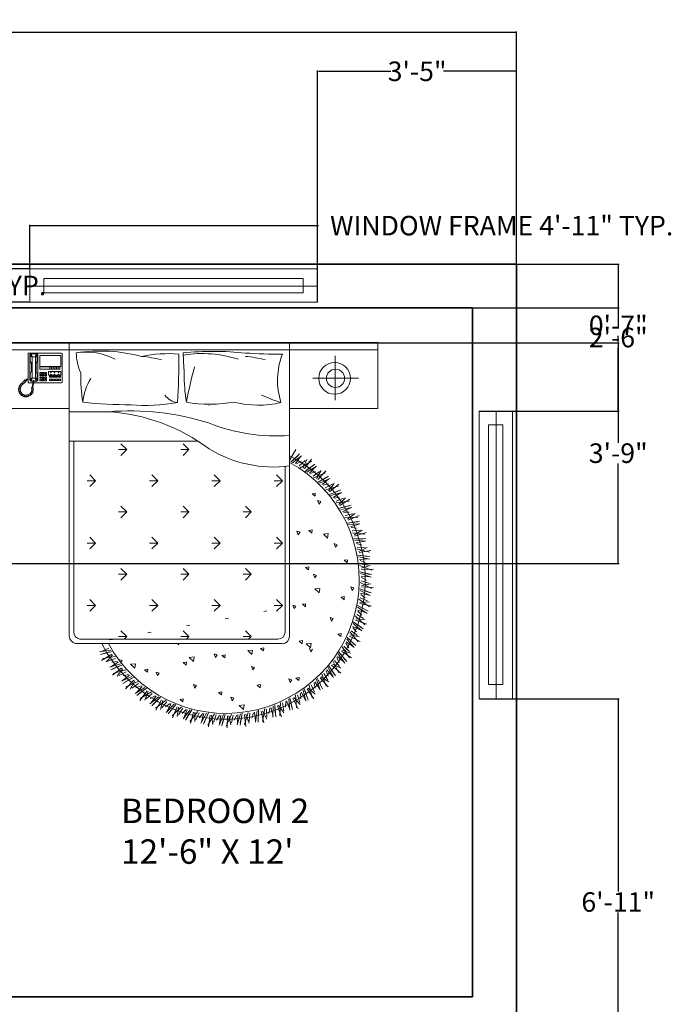
# Model space of a CAD drawing. Units: inches. Extents: x 311 to 754, y 60 to 497.
# Tile 11 of 11: x 621 to 754, y 296 to 497. Entities that reach past the tile are written whole.
import ezdxf

# ---------------------------------------------------------------- set-up
doc = ezdxf.new("R2010")
doc.units = ezdxf.units.IN
doc.header["$MEASUREMENT"] = 0
for name, color, linetype, lineweight in [('A-ANNO-DIMS', 2, 'Continuous', 18), ('A-AREA-IDEN', 1, 'Continuous', 18), ('A-WALL', 7, 'Continuous', 35), ('beds', 70, 'Continuous', 13), ('windows', 120, 'Continuous', 18)]:
    doc.layers.add(name, color=color, linetype=linetype, lineweight=lineweight)
doc.styles.get("Standard").update_dxf_attribs({"font": 'arial.ttf'})
doc.dimstyles.get("Standard").update_dxf_attribs({"dimtxt": 4, "dimasz": 0.18, "dimexe": 0.18, "dimexo": 0.0625, "dimgap": 0.09, "dimtad": 0, "dimtih": 1, "dimtoh": 1, "dimdec": 0, "dimrnd": 6, "dimzin": 0, "dimdsep": 46, "dimlunit": 3, "dimtxsty": 'Standard', "dimcen": 0.09, "dimadec": 0, "dimazin": 0, "dimtfac": 1, "dimtdec": 0, "dimtofl": 0, "dimtmove": 0, "dimatfit": 3, "dimfxl": 1, "dimtolj": 1, "dimtzin": 0, "dimarcsym": 0})

# ---------------------------------------------------------------- blocks, each defined once
blk = doc.blocks.new('A$C57792D97')
for p, q in [((0.6, 2.6235), (0, 2.6235)), ((0, 2.6235), (0, 2.1735)), ((2.1, 2.6235), (0.6, 2.6235)), ((0.6, 2.6235), (0.6, 0.6235)), ((0.6, 0.6235), (0.6, 2.6235)), ((0.6, 2.1735), (0.6, 2.6235)), ((2.1, 0.6235), (2.1, 2.6235)), ((2.7, 2.6235), (2.1, 2.6235)), ((2.1, 2.6235), (2.1, 2.1735)), ((2.7, 2.1735), (2.7, 2.6235)), ((0.6, 2.5735), (0, 2.5735)), ((2.1, 2.5735), (0.6, 2.5735)), ((2.7, 2.5735), (2.1, 2.5735)), ((2.4103, 2.2312), (2.4103, 2.5317)), ((2.2593, 2.3802), (2.5698, 2.3802)), ((0, 2.1735), (0.6, 2.1735)), ((0.6, 2.1518), (0.8661, 2.1518)), ((1.5491, 2.1955), (1.5516, 2.1955)), ((2.1, 2.1735), (2.7, 2.1735)), ((0.6, 1.9518), (1.4767, 1.9518)), ((0.63, 0.6535), (0.63, 1.9518)), ((0.9906, 1.8942), (0.9344, 1.8942)), ((0.9906, 1.8942), (0.9508, 1.934)), ((0.9906, 1.8942), (0.9508, 1.8544)), ((1.4149, 1.8942), (1.3586, 1.8942)), ((1.4149, 1.8942), (1.3751, 1.934)), ((1.4149, 1.8942), (1.3751, 1.8544)), ((2.142, 1.8959), (2.1018, 1.8254)), ((2.1679, 1.8652), (2.1088, 1.8077)), ((2.1584, 1.8544), (2.1201, 1.8188)), ((2.1812, 1.8524), (2.1207, 1.8046)), ((2.1749, 1.8475), (2.1394, 1.7993)), ((2.1799, 1.8155), (2.1465, 1.7971)), ((2.2066, 1.8191), (2.1664, 1.7827)), ((2.249, 1.8154), (2.1711, 1.7709)), ((2.2173, 1.8274), (2.1931, 1.7688)), ((2.2496, 1.8292), (2.2008, 1.7642)), ((2.07, 1.7793), (2.07, 0.6535)), ((2.2713, 1.7954), (2.2055, 1.7458)), ((2.283, 1.7811), (2.2169, 1.7413)), ((2.2607, 1.7859), (2.2181, 1.7554)), ((2.2761, 1.777), (2.2348, 1.7337)), ((2.277, 1.7446), (2.2416, 1.7306)), ((2.304, 1.7449), (2.2596, 1.7138)), ((2.3157, 1.7518), (2.2843, 1.6966)), ((2.3479, 1.7495), (2.2914, 1.6911)), ((0.7785, 1.6821), (0.7222, 1.6821)), ((0.7785, 1.6821), (0.7387, 1.7219)), ((0.7785, 1.6821), (0.7387, 1.6423)), ((1.2027, 1.6821), (1.1465, 1.6821)), ((1.2027, 1.6821), (1.163, 1.7219)), ((1.2027, 1.6821), (1.163, 1.6423)), ((1.627, 1.6821), (1.5708, 1.6821)), ((1.627, 1.6821), (1.5872, 1.7219)), ((1.627, 1.6821), (1.5872, 1.6423)), ((2.0513, 1.6821), (1.995, 1.6821)), ((2.0513, 1.6821), (2.0115, 1.7219)), ((2.0513, 1.6821), (2.0115, 1.6423)), ((2.3456, 1.7359), (2.2627, 1.7015)), ((2.3653, 1.7133), (2.2937, 1.6723)), ((2.3751, 1.6976), (2.3045, 1.6664)), ((2.3535, 1.7051), (2.3075, 1.6802)), ((2.3677, 1.6944), (2.3213, 1.6565)), ((2.3645, 1.6621), (2.3277, 1.6526)), ((2.3913, 1.659), (2.3434, 1.6337)), ((2.4314, 1.6449), (2.3449, 1.6211)), ((2.4038, 1.6644), (2.3657, 1.6136)), ((2.4355, 1.6581), (2.372, 1.6073)), ((2.4482, 1.62), (2.372, 1.5882)), ((2.4354, 1.6134), (2.3867, 1.5944)), ((2.2754, 1.598), (2.2534, 1.5939)), ((2.2736, 1.5771), (2.2535, 1.594)), ((2.2736, 1.5771), (2.2754, 1.598)), ((2.3123, 1.541), (2.2911, 1.5481)), ((2.3006, 1.5236), (2.2912, 1.5481)), ((2.4559, 1.6032), (2.382, 1.581)), ((2.4482, 1.6009), (2.3974, 1.5692)), ((2.441, 1.5693), (2.4032, 1.5645)), ((2.4672, 1.5629), (2.4164, 1.5438)), ((2.5052, 1.5438), (2.4164, 1.5311)), ((2.4802, 1.5667), (2.4361, 1.5211)), ((2.5109, 1.5564), (2.4416, 1.514)), ((0.9906, 1.47), (0.9508, 1.5097)), ((1.4149, 1.47), (1.3751, 1.5097)), ((1.8391, 1.47), (1.7994, 1.5097)), ((2.3006, 1.5236), (2.3123, 1.541)), ((2.5187, 1.517), (2.4392, 1.4951)), ((2.5243, 1.4994), (2.4482, 1.4867)), ((2.5052, 1.5121), (2.4545, 1.4994)), ((2.5163, 1.4981), (2.462, 1.473)), ((0.9906, 1.47), (0.9344, 1.47)), ((0.9906, 1.47), (0.9508, 1.4302)), ((1.4149, 1.47), (1.3586, 1.47)), ((1.4149, 1.47), (1.3751, 1.4302)), ((1.8391, 1.47), (1.7829, 1.47)), ((1.8391, 1.47), (1.7994, 1.4302)), ((2.5052, 1.4677), (2.4672, 1.4677)), ((2.5658, 1.4343), (2.4761, 1.4328)), ((2.5304, 1.458), (2.4777, 1.4454)), ((2.5438, 1.4601), (2.4943, 1.4204)), ((2.573, 1.4461), (2.4989, 1.4127)), ((2.2534, 1.3469), (2.2315, 1.3429)), ((2.2516, 1.326), (2.2315, 1.3429)), ((2.2516, 1.326), (2.2535, 1.347)), ((2.5758, 1.406), (2.4942, 1.3942)), ((2.5791, 1.3878), (2.502, 1.3848)), ((2.5618, 1.4028), (2.5099, 1.3966)), ((2.571, 1.3876), (2.514, 1.3695)), ((2.5562, 1.3587), (2.5185, 1.3635)), ((2.58, 1.346), (2.5261, 1.3402)), ((2.5936, 1.3464), (2.5395, 1.3132)), ((0.7785, 1.2578), (0.7387, 1.2976)), ((1.2027, 1.2578), (1.163, 1.2976)), ((1.627, 1.2578), (1.5872, 1.2976)), ((2.0513, 1.2578), (2.0115, 1.2976)), ((2.1596, 1.3147), (2.1502, 1.3392)), ((2.1714, 1.3321), (2.1502, 1.3392)), ((2.1596, 1.3147), (2.1714, 1.3321)), ((2.3632, 1.3229), (2.33, 1.319)), ((2.3584, 1.2918), (2.33, 1.319)), ((2.3584, 1.2918), (2.3632, 1.3229)), ((2.6121, 1.3181), (2.523, 1.3279)), ((2.6185, 1.2888), (2.5361, 1.2873)), ((2.6195, 1.2703), (2.5426, 1.277)), ((2.6207, 1.3289), (2.5431, 1.305)), ((2.6042, 1.2873), (2.5519, 1.2877)), ((0.7785, 1.2578), (0.7222, 1.2578)), ((0.7785, 1.2578), (0.7387, 1.218)), ((1.2027, 1.2578), (1.1465, 1.2578)), ((1.2027, 1.2578), (1.163, 1.218)), ((1.627, 1.2578), (1.5708, 1.2578)), ((1.627, 1.2578), (1.5872, 1.218)), ((2.0513, 1.2578), (1.995, 1.2578)), ((2.0513, 1.2578), (2.0115, 1.218)), ((2.4134, 1.2295), (2.404, 1.254)), ((2.4252, 1.2469), (2.404, 1.254)), ((2.4134, 1.2295), (2.4252, 1.2469)), ((2.6115, 1.2711), (2.5526, 1.2603)), ((2.5932, 1.2443), (2.5563, 1.2538)), ((2.6435, 1.197), (2.5563, 1.2178)), ((2.6152, 1.2287), (2.561, 1.2296)), ((2.6287, 1.2274), (2.5709, 1.2013)), ((2.4947, 1.1445), (2.4728, 1.1404)), ((2.4929, 1.1236), (2.4728, 1.1404)), ((2.4929, 1.1236), (2.4948, 1.1445)), ((2.6462, 1.1671), (2.5642, 1.176)), ((2.6449, 1.1486), (2.5694, 1.1649)), ((2.6534, 1.2066), (2.5734, 1.1926)), ((2.637, 1.1504), (2.5773, 1.147)), ((2.6319, 1.1675), (2.58, 1.1743)), ((2.6155, 1.1261), (2.5801, 1.1402)), ((0.9906, 1.0457), (0.9508, 1.0855)), ((1.4149, 1.0457), (1.3751, 1.0855)), ((1.8391, 1.0457), (1.7994, 1.0855)), ((2.2315, 1.0959), (2.2095, 1.0919)), ((2.2297, 1.075), (2.2096, 1.0919)), ((2.2297, 1.075), (2.2315, 1.0959)), ((2.6595, 1.0729), (2.5756, 1.1045)), ((2.6353, 1.1079), (2.5817, 1.1156)), ((2.6486, 1.1049), (2.588, 1.0862)), ((2.6705, 1.0812), (2.5894, 1.0774)), ((0.9906, 1.0457), (0.9344, 1.0457)), ((0.9906, 1.0457), (0.9508, 1.0059)), ((1.4149, 1.0457), (1.3586, 1.0457)), ((1.4149, 1.0457), (1.3751, 1.0059)), ((1.8391, 1.0457), (1.7829, 1.0457)), ((1.8391, 1.0457), (1.7994, 1.0059)), ((2.2725, 1.0206), (2.2631, 1.0451)), ((2.2842, 1.038), (2.2631, 1.0451)), ((2.2725, 1.0206), (2.2843, 1.038)), ((2.6584, 1.0429), (2.5782, 1.062)), ((2.6548, 1.0248), (2.582, 1.0503)), ((2.6472, 1.0275), (2.5875, 1.0316)), ((2.6228, 1.0061), (2.5895, 1.0244)), ((2.6442, 1.045), (2.5937, 1.0584)), ((2.3053, 0.9493), (2.272, 0.9455)), ((2.3005, 0.9182), (2.2721, 0.9455)), ((2.3005, 0.9182), (2.3053, 0.9494)), ((2.5263, 0.9355), (2.5169, 0.96)), ((2.538, 0.9528), (2.5169, 0.9599)), ((2.5263, 0.9355), (2.5381, 0.9529)), ((2.655, 0.9181), (2.5778, 0.9471)), ((2.6598, 0.9477), (2.5805, 0.9897)), ((2.6402, 0.9855), (2.588, 0.9999)), ((2.653, 0.9809), (2.5905, 0.97)), ((2.6718, 0.9546), (2.5908, 0.961)), ((2.6412, 0.9221), (2.5927, 0.9416)), ((0.7785, 0.8336), (0.7387, 0.8733)), ((1.2027, 0.8336), (1.163, 0.8733)), ((1.627, 0.8336), (1.5872, 0.8733)), ((2.0513, 0.8336), (2.0115, 0.8733)), ((2.4728, 0.8934), (2.4508, 0.8894)), ((2.471, 0.8725), (2.4509, 0.8894)), ((2.471, 0.8725), (2.4728, 0.8934)), ((2.6444, 0.8236), (2.571, 0.8751)), ((2.6297, 0.8635), (2.5797, 0.8843)), ((2.6491, 0.9006), (2.5801, 0.9351)), ((2.6419, 0.9043), (2.5832, 0.9159)), ((2.6151, 0.8861), (2.5843, 0.9085)), ((0.7785, 0.8336), (0.7222, 0.8336)), ((0.7785, 0.8336), (0.7387, 0.7938)), ((1.2027, 0.8336), (1.1465, 0.8336)), ((1.2027, 0.8336), (1.163, 0.7938)), ((1.627, 0.8336), (1.5708, 0.8336)), ((1.627, 0.8336), (1.5872, 0.7938)), ((2.0513, 0.8336), (1.995, 0.8336)), ((2.0513, 0.8336), (2.0115, 0.7938)), ((2.1316, 0.8117), (2.1222, 0.8362)), ((2.1433, 0.8291), (2.1222, 0.8362)), ((2.1316, 0.8117), (2.1434, 0.8291)), ((2.2095, 0.8449), (2.1876, 0.8408)), ((2.2077, 0.824), (2.1876, 0.8408)), ((2.2077, 0.824), (2.2095, 0.8449)), ((2.6359, 0.7948), (2.5629, 0.8332)), ((2.6279, 0.7781), (2.5637, 0.821)), ((2.6227, 0.8004), (2.577, 0.8259)), ((2.6572, 0.8289), (2.5776, 0.8454)), ((2.6418, 0.8573), (2.5785, 0.8543)), ((1.683, 0.7477), (1.661, 0.7437)), ((1.9462, 0.7963), (1.9243, 0.7923)), ((2.3854, 0.7265), (2.376, 0.751)), ((2.3971, 0.7439), (2.376, 0.751)), ((2.3854, 0.7265), (2.3972, 0.7439)), ((2.6136, 0.7023), (2.5472, 0.7626)), ((2.6153, 0.7361), (2.552, 0.7411)), ((2.604, 0.7437), (2.557, 0.7707)), ((2.6212, 0.7827), (2.5644, 0.8015)), ((2.5923, 0.768), (2.5646, 0.7941)), ((1.4197, 0.6992), (1.3978, 0.6951)), ((2.5549, 0.6537), (2.5307, 0.6831)), ((2.5855, 0.6646), (2.5315, 0.6905)), ((2.5915, 0.6593), (2.5332, 0.7099)), ((2.6016, 0.6748), (2.534, 0.7221)), ((2.5892, 0.6821), (2.547, 0.7131)), ((2.6269, 0.706), (2.5501, 0.7323)), ((2.02, 0.6035), (0.6716, 0.6035)), ((0.9906, 0.6214), (0.9344, 0.6214)), ((0.9906, 0.6214), (0.9508, 0.6612)), ((0.9906, 0.6214), (0.9727, 0.6035)), ((1.1564, 0.6506), (1.1345, 0.6466)), ((1.4149, 0.6214), (1.3586, 0.6214)), ((1.4149, 0.6214), (1.3751, 0.6612)), ((1.4149, 0.6214), (1.397, 0.6035)), ((1.8391, 0.6214), (1.7829, 0.6214)), ((1.8391, 0.6214), (1.7994, 0.6612)), ((1.8391, 0.6214), (1.8212, 0.6035)), ((2.4508, 0.6424), (2.4289, 0.6383)), ((2.449, 0.6215), (2.4289, 0.6384)), ((2.449, 0.6215), (2.4508, 0.6424)), ((2.5405, 0.546), (2.489, 0.6034)), ((2.5524, 0.5601), (2.4913, 0.6155)), ((2.541, 0.5688), (2.5031, 0.6049)), ((2.5815, 0.5878), (2.5085, 0.6236)), ((2.5678, 0.5858), (2.5095, 0.654)), ((2.5737, 0.6192), (2.5116, 0.632)), ((2.5635, 0.6282), (2.5203, 0.6608)), ((0.6417, 0.5735), (2.05, 0.5735)), ((0.8142, 0.5177), (0.8685, 0.5428)), ((0.8932, 0.6021), (0.8712, 0.598)), ((1.3422, 0.5642), (1.3386, 0.5735)), ((1.3422, 0.5642), (1.3485, 0.5735)), ((1.9243, 0.5453), (1.9023, 0.5412)), ((1.9225, 0.5244), (1.9024, 0.5412)), ((1.9225, 0.5244), (1.9243, 0.5453)), ((2.1875, 0.5938), (2.1656, 0.5898)), ((2.1857, 0.5729), (2.1656, 0.5898)), ((2.1857, 0.5729), (2.1876, 0.5938)), ((2.2473, 0.5758), (2.2141, 0.5719)), ((2.2425, 0.5447), (2.2141, 0.572)), ((2.2445, 0.5176), (2.2351, 0.5421)), ((2.2425, 0.5447), (2.2474, 0.5758)), ((2.5078, 0.476), (2.4585, 0.551)), ((2.5088, 0.5186), (2.47, 0.5564)), ((2.5035, 0.545), (2.4831, 0.5772)), ((2.5352, 0.552), (2.4849, 0.5844)), ((0.8062, 0.5164), (0.8823, 0.5291)), ((0.8118, 0.4988), (0.8913, 0.5207)), ((0.8196, 0.4594), (0.8889, 0.5018)), ((0.8253, 0.5037), (0.876, 0.5164)), ((0.8253, 0.472), (0.9141, 0.4847)), ((0.8503, 0.4491), (0.8944, 0.4947)), ((0.8633, 0.4529), (0.9141, 0.472)), ((1.4496, 0.483), (1.4163, 0.4791)), ((1.4448, 0.4519), (1.4164, 0.4792)), ((1.4448, 0.4519), (1.4496, 0.483)), ((1.6077, 0.4964), (1.5865, 0.5035)), ((1.596, 0.479), (1.5866, 0.5035)), ((1.596, 0.479), (1.6077, 0.4964)), ((1.661, 0.4967), (1.6391, 0.4927)), ((1.6592, 0.4758), (1.6391, 0.4927)), ((1.6592, 0.4758), (1.661, 0.4967)), ((1.8485, 0.5294), (1.8152, 0.5255)), ((1.8437, 0.4983), (1.8153, 0.5256)), ((1.8437, 0.4983), (1.8485, 0.5294)), ((2.2445, 0.5176), (2.2562, 0.535)), ((2.4389, 0.4436), (2.4227, 0.478)), ((2.4712, 0.4466), (2.4253, 0.485)), ((2.4757, 0.4399), (2.4318, 0.5034)), ((2.4893, 0.4525), (2.4356, 0.515)), ((2.4791, 0.4625), (2.446, 0.503)), ((2.5216, 0.4763), (2.4537, 0.5209)), ((2.5178, 0.5084), (2.4578, 0.5289)), ((0.8746, 0.4126), (0.9485, 0.4347)), ((0.8823, 0.4149), (0.9331, 0.4466)), ((0.8823, 0.3958), (0.9585, 0.4275)), ((0.8895, 0.4465), (0.9273, 0.4513)), ((0.895, 0.3577), (0.9585, 0.4085)), ((0.8951, 0.4024), (0.9438, 0.4214)), ((0.9592, 0.4578), (0.938, 0.4649)), ((0.9403, 0.459), (0.9381, 0.4649)), ((0.9508, 0.4454), (0.9592, 0.4578)), ((1.0507, 0.4366), (1.0175, 0.4327)), ((1.0459, 0.4055), (1.0175, 0.4328)), ((1.0459, 0.4055), (1.0507, 0.4366)), ((1.3977, 0.4481), (1.3758, 0.4441)), ((1.3959, 0.4272), (1.3758, 0.4441)), ((1.3959, 0.4272), (1.3978, 0.4482)), ((1.8615, 0.4113), (1.8403, 0.4184)), ((1.8498, 0.3939), (1.8404, 0.4184)), ((1.8498, 0.3939), (1.8615, 0.4113)), ((2.3981, 0.3428), (2.3625, 0.4113)), ((2.4132, 0.3535), (2.3678, 0.4224)), ((2.4043, 0.3648), (2.3766, 0.4092)), ((2.4482, 0.3731), (2.3865, 0.4259)), ((2.4485, 0.4055), (2.3915, 0.4334)), ((2.4345, 0.3746), (2.395, 0.4552)), ((2.4409, 0.4167), (2.4071, 0.4591)), ((0.8991, 0.3709), (0.9856, 0.3946)), ((0.9267, 0.3514), (0.9648, 0.4022)), ((0.9392, 0.3568), (0.9872, 0.3821)), ((0.9555, 0.3182), (1.026, 0.3494)), ((0.9628, 0.3214), (1.0092, 0.3592)), ((0.9652, 0.3025), (1.0368, 0.3435)), ((0.966, 0.3537), (1.0029, 0.3631)), ((0.977, 0.3107), (1.023, 0.3356)), ((1.1345, 0.3996), (1.1125, 0.3955)), ((1.1327, 0.3787), (1.1126, 0.3955)), ((1.1327, 0.3787), (1.1345, 0.3996)), ((1.213, 0.3727), (1.1918, 0.3798)), ((1.2013, 0.3553), (1.1919, 0.3798)), ((1.2013, 0.3553), (1.213, 0.3727)), ((2.1656, 0.3428), (2.1436, 0.3387)), ((2.1638, 0.3219), (2.1437, 0.3388)), ((2.1638, 0.3219), (2.1656, 0.3428)), ((2.3253, 0.265), (2.2888, 0.3389)), ((2.3625, 0.28), (2.3078, 0.3401)), ((2.3668, 0.3121), (2.3138, 0.3469)), ((2.3491, 0.2832), (2.32, 0.3681)), ((2.3607, 0.3242), (2.3324, 0.3704)), ((2.3621, 0.3511), (2.3503, 0.3873)), ((2.3945, 0.35), (2.3538, 0.3939)), ((0.9826, 0.2663), (1.0392, 0.3246)), ((0.9849, 0.2799), (1.0678, 0.3143)), ((1.0148, 0.264), (1.0462, 0.3191)), ((1.0265, 0.2709), (1.0709, 0.302)), ((1.0475, 0.2347), (1.1136, 0.2745)), ((1.0535, 0.2712), (1.0889, 0.2852)), ((1.0544, 0.2388), (1.0957, 0.2821)), ((1.0592, 0.2203), (1.125, 0.27)), ((1.4668, 0.2875), (1.4456, 0.2946)), ((1.4551, 0.2701), (1.4457, 0.2946)), ((1.4551, 0.2701), (1.4668, 0.2875)), ((1.9023, 0.2942), (1.8804, 0.2902)), ((1.9005, 0.2733), (1.8804, 0.2902)), ((1.9005, 0.2733), (1.9023, 0.2942)), ((2.1153, 0.3261), (2.0941, 0.3332)), ((2.1036, 0.3087), (2.0942, 0.3332)), ((2.1036, 0.3087), (2.1153, 0.3261)), ((2.2741, 0.2296), (2.2258, 0.2708)), ((2.2529, 0.2032), (2.2346, 0.291)), ((2.2695, 0.2424), (2.2473, 0.2918)), ((2.2743, 0.2689), (2.2671, 0.3063)), ((2.3063, 0.2638), (2.2714, 0.3124)), ((2.309, 0.2562), (2.2823, 0.3286)), ((2.3179, 0.2773), (2.2959, 0.3247)), ((1.0699, 0.2299), (1.1124, 0.2604)), ((1.0809, 0.1866), (1.1297, 0.2516)), ((1.0815, 0.2004), (1.1594, 0.2449)), ((1.1132, 0.1884), (1.1374, 0.247)), ((1.1239, 0.1967), (1.1641, 0.2331)), ((1.1493, 0.1634), (1.2098, 0.2112)), ((1.1507, 0.2003), (1.184, 0.2187)), ((1.1556, 0.1683), (1.1911, 0.2165)), ((1.1626, 0.1506), (1.2217, 0.2081)), ((1.639, 0.2457), (1.6171, 0.2416)), ((1.6372, 0.2248), (1.6171, 0.2416)), ((1.6372, 0.2248), (1.6391, 0.2457)), ((1.7206, 0.2023), (1.6994, 0.2094)), ((1.7089, 0.1849), (1.6995, 0.2095)), ((1.7089, 0.1849), (1.7206, 0.2024)), ((2.1198, 0.1242), (2.1029, 0.2049)), ((2.1596, 0.1295), (2.1216, 0.2013)), ((2.1718, 0.1594), (2.129, 0.2063)), ((2.1474, 0.1359), (2.1403, 0.2253)), ((2.1688, 0.1727), (2.1529, 0.2245)), ((2.1768, 0.1984), (2.1745, 0.2364)), ((2.208, 0.1893), (2.1795, 0.2419)), ((2.2097, 0.1814), (2.1923, 0.2566)), ((2.227, 0.1881), (2.2001, 0.2661)), ((2.2212, 0.2012), (2.2053, 0.2511)), ((2.2658, 0.1984), (2.2191, 0.2649)), ((1.1721, 0.1614), (1.2104, 0.197)), ((1.1873, 0.1336), (1.259, 0.1875)), ((1.1885, 0.1199), (1.2287, 0.1904)), ((1.2203, 0.1256), (1.237, 0.1868)), ((1.2299, 0.1352), (1.2652, 0.1764)), ((1.2559, 0.1422), (1.2867, 0.1646)), ((1.2592, 0.1054), (1.3133, 0.1604)), ((1.2649, 0.111), (1.2941, 0.1633)), ((1.2741, 0.0944), (1.3255, 0.1588)), ((1.282, 0.1063), (1.3156, 0.1464)), ((1.3007, 0.0806), (1.3651, 0.1431)), ((1.3035, 0.0671), (1.3346, 0.1421)), ((1.3344, 0.0768), (1.3433, 0.1396)), ((1.3758, 0.1971), (1.3538, 0.193)), ((1.374, 0.1762), (1.3539, 0.1931)), ((1.374, 0.1762), (1.3758, 0.1971)), ((1.7905, 0.1559), (1.7573, 0.152)), ((1.7857, 0.1248), (1.7573, 0.152)), ((1.7857, 0.1248), (1.7906, 0.1559)), ((1.9873, 0.08), (1.9728, 0.1381)), ((1.9871, 0.072), (1.9889, 0.1491)), ((2.0054, 0.0742), (1.9988, 0.1564)), ((2.0031, 0.0883), (2.0001, 0.1405)), ((2.0456, 0.0745), (2.0169, 0.1505)), ((2.0614, 0.1027), (2.0249, 0.1545)), ((2.0343, 0.0824), (2.0385, 0.172)), ((2.0601, 0.1162), (2.0509, 0.1696)), ((2.0714, 0.1407), (2.0737, 0.1787)), ((2.1011, 0.1277), (2.0794, 0.1835)), ((2.1018, 0.1197), (2.0939, 0.1965)), ((2.1157, 0.1379), (2.1062, 0.1893)), ((1.3427, 0.0876), (1.3725, 0.1328)), ((1.3677, 0.0977), (1.3954, 0.1238)), ((1.3755, 0.0616), (1.4223, 0.1229)), ((1.3804, 0.0679), (1.4028, 0.1234)), ((1.3916, 0.0525), (1.4346, 0.1229)), ((1.3981, 0.0653), (1.4264, 0.1093)), ((1.4198, 0.0422), (1.4758, 0.1123)), ((1.4243, 0.0292), (1.4458, 0.1075)), ((1.4537, 0.0427), (1.4546, 0.1061)), ((1.4606, 0.0544), (1.4845, 0.103)), ((1.4841, 0.0676), (1.5083, 0.0969)), ((1.4964, 0.0327), (1.5351, 0.0995)), ((1.5005, 0.0397), (1.5158, 0.0975)), ((1.5135, 0.0258), (1.5473, 0.101)), ((1.5183, 0.0393), (1.5409, 0.0865)), ((1.5428, 0.0191), (1.5896, 0.0956)), ((1.5489, 0.0067), (1.5603, 0.0871)), ((1.5763, 0.0238), (1.5693, 0.0868)), ((1.5817, 0.0362), (1.5994, 0.0875)), ((1.6034, 0.0523), (1.6237, 0.0845)), ((1.6199, 0.0192), (1.65, 0.0903)), ((1.6232, 0.0266), (1.631, 0.086)), ((1.6378, 0.0145), (1.6619, 0.0934)), ((1.6409, 0.0285), (1.6573, 0.0782)), ((1.6677, 0.0115), (1.7045, 0.0933)), ((1.6753, 0), (1.6766, 0.0812)), ((1.7004, 0.0204), (1.6855, 0.0821)), ((1.7041, 0.0334), (1.7152, 0.0865)), ((1.7236, 0.0521), (1.7398, 0.0865)), ((1.7442, 0.0214), (1.7651, 0.0956)), ((1.7465, 0.0291), (1.7469, 0.0889)), ((1.7625, 0.0189), (1.7765, 0.1002)), ((1.7638, 0.0332), (1.7739, 0.0845)), ((1.7925, 0.0197), (1.8188, 0.1054)), ((1.8015, 0.0092), (1.7926, 0.09)), ((1.8238, 0.0326), (1.8014, 0.0919)), ((1.8259, 0.046), (1.8303, 0.1)), ((1.8429, 0.0669), (1.8547, 0.1031)), ((1.8685, 0.047), (1.8614, 0.1064)), ((1.8672, 0.039), (1.8787, 0.1154)), ((1.8852, 0.0532), (1.8888, 0.1054)), ((1.8857, 0.0389), (1.8894, 0.1213)), ((1.9256, 0.0342), (1.9067, 0.1132)), ((1.9448, 0.0601), (1.9151, 0.1162)), ((1.9154, 0.0434), (1.9307, 0.1318)), ((1.9452, 0.0737), (1.9428, 0.1279)), ((1.9595, 0.0966), (1.9666, 0.134))]:
    blk.add_line(p, q)
at = {"linetype": 'ByBlock'}
for p, q in [((0.3217, 2.5511), (0.3189, 2.5483)), ((0.3189, 2.5483), (0.3189, 2.3511)), ((0.5475, 2.5511), (0.3217, 2.5511)), ((0.5475, 2.5511), (0.5503, 2.5483)), ((0.5503, 2.5483), (0.5503, 2.3511)), ((0.3375, 2.5469), (0.3303, 2.5397)), ((0.3303, 2.5397), (0.3303, 2.3683)), ((0.3346, 2.5426), (0.3332, 2.5369)), ((0.3332, 2.5369), (0.3332, 2.4983)), ((0.3332, 2.5369), (0.346, 2.524)), ((0.3332, 2.4983), (0.336, 2.4911)), ((0.3403, 2.5454), (0.3346, 2.5426)), ((0.336, 2.4911), (0.3403, 2.484)), ((0.3803, 2.5469), (0.3375, 2.5469)), ((0.3746, 2.5454), (0.3403, 2.5454)), ((0.3475, 2.5269), (0.3403, 2.5454)), ((0.3403, 2.484), (0.3417, 2.474)), ((0.346, 2.524), (0.3475, 2.5269)), ((0.346, 2.4597), (0.346, 2.524)), ((0.3475, 2.5269), (0.3675, 2.5269)), ((0.3675, 2.5269), (0.3746, 2.5454)), ((0.3689, 2.524), (0.3675, 2.5269)), ((0.3818, 2.5369), (0.3689, 2.524)), ((0.3689, 2.4597), (0.3689, 2.524)), ((0.3746, 2.484), (0.3732, 2.474)), ((0.3746, 2.5454), (0.3803, 2.5426)), ((0.3789, 2.4911), (0.3746, 2.484)), ((0.3818, 2.4983), (0.3789, 2.4911)), ((0.386, 2.5397), (0.3803, 2.5469)), ((0.3803, 2.5426), (0.3818, 2.5369)), ((0.3818, 2.5369), (0.3818, 2.4983)), ((0.386, 2.3668), (0.386, 2.5397)), ((0.3989, 2.4597), (0.3989, 2.5354)), ((0.3989, 2.5354), (0.5418, 2.5354)), ((0.5418, 2.5354), (0.5418, 2.4597)), ((0.3332, 2.4083), (0.336, 2.4154)), ((0.336, 2.4154), (0.3403, 2.4226)), ((0.3403, 2.4226), (0.3417, 2.4326)), ((0.3417, 2.474), (0.3417, 2.4597)), ((0.3417, 2.4326), (0.3417, 2.4597)), ((0.346, 2.4597), (0.346, 2.3826)), ((0.3689, 2.4597), (0.3689, 2.3826)), ((0.3732, 2.474), (0.3732, 2.4597)), ((0.3732, 2.4326), (0.3732, 2.4597)), ((0.3746, 2.4226), (0.3732, 2.4326)), ((0.3789, 2.4154), (0.3746, 2.4226)), ((0.3818, 2.4083), (0.3789, 2.4154)), ((0.5418, 2.4597), (0.3989, 2.4597)), ((0.3989, 2.4426), (0.3989, 2.4568)), ((0.3989, 2.4568), (0.5361, 2.4568)), ((0.5361, 2.4426), (0.3989, 2.4426)), ((0.3989, 2.4197), (0.3989, 2.4111)), ((0.4103, 2.4197), (0.3989, 2.4197)), ((0.4103, 2.4111), (0.4103, 2.4197)), ((0.4275, 2.4197), (0.416, 2.4197)), ((0.416, 2.4197), (0.416, 2.4111)), ((0.4275, 2.4111), (0.4275, 2.4197)), ((0.4332, 2.4197), (0.4332, 2.4111)), ((0.4446, 2.4197), (0.4332, 2.4197)), ((0.4446, 2.4111), (0.4446, 2.4197)), ((0.4575, 2.4011), (0.4575, 2.4268)), ((0.4575, 2.4268), (0.5418, 2.4268)), ((0.4675, 2.4568), (0.4675, 2.4426)), ((0.4718, 2.424), (0.4761, 2.424)), ((0.4718, 2.4197), (0.4718, 2.424)), ((0.4761, 2.4197), (0.4718, 2.4197)), ((0.4761, 2.424), (0.4761, 2.4197)), ((0.4789, 2.4568), (0.4789, 2.4426)), ((0.4903, 2.4568), (0.4903, 2.4426)), ((0.4975, 2.424), (0.5018, 2.424)), ((0.4975, 2.4197), (0.4975, 2.424)), ((0.5018, 2.4197), (0.4975, 2.4197)), ((0.5018, 2.4568), (0.5018, 2.4426)), ((0.5018, 2.424), (0.5018, 2.4197)), ((0.5132, 2.4568), (0.5132, 2.4426)), ((0.5232, 2.4197), (0.5232, 2.424)), ((0.5232, 2.424), (0.5275, 2.424)), ((0.5275, 2.4197), (0.5232, 2.4197)), ((0.5246, 2.4568), (0.5246, 2.4426)), ((0.5275, 2.424), (0.5275, 2.4197)), ((0.5361, 2.4568), (0.5361, 2.4426)), ((0.5418, 2.4268), (0.5418, 2.4011)), ((0.2937, 2.3497), (0.2748, 2.3336)), ((0.2789, 2.3502), (0.2854, 2.3565)), ((0.2804, 2.3412), (0.2789, 2.3502)), ((0.2854, 2.3565), (0.2932, 2.3525)), ((0.2902, 2.3608), (0.294, 2.3648)), ((0.2932, 2.3525), (0.2902, 2.3608)), ((0.3053, 2.3601), (0.2937, 2.3497)), ((0.294, 2.3648), (0.2975, 2.3621)), ((0.2955, 2.3663), (0.298, 2.3689)), ((0.2975, 2.3621), (0.2955, 2.3663)), ((0.298, 2.3689), (0.3033, 2.3669)), ((0.3053, 2.3628), (0.3023, 2.3631)), ((0.3023, 2.3631), (0.3053, 2.3601)), ((0.3033, 2.3669), (0.3063, 2.3696)), ((0.3068, 2.3648), (0.3053, 2.3628)), ((0.3063, 2.3696), (0.3103, 2.3737)), ((0.3126, 2.3694), (0.3068, 2.3648)), ((0.3103, 2.3737), (0.3189, 2.3768)), ((0.3189, 2.3711), (0.3126, 2.3694)), ((0.3189, 2.3511), (0.3217, 2.3483)), ((0.3217, 2.3483), (0.3525, 2.3483)), ((0.3303, 2.3683), (0.3375, 2.3597)), ((0.3332, 2.3697), (0.3332, 2.4083)), ((0.3332, 2.3697), (0.346, 2.3826)), ((0.3346, 2.364), (0.3332, 2.3697)), ((0.3403, 2.3611), (0.3346, 2.364)), ((0.3375, 2.3597), (0.3542, 2.3597)), ((0.3475, 2.3797), (0.3403, 2.3611)), ((0.3543, 2.3611), (0.3403, 2.3611)), ((0.346, 2.3826), (0.3475, 2.3797)), ((0.3475, 2.3797), (0.3675, 2.3797)), ((0.3518, 2.3447), (0.3538, 2.354)), ((0.3538, 2.354), (0.3546, 2.3654)), ((0.3546, 2.3654), (0.3589, 2.3654)), ((0.3587, 2.3531), (0.3552, 2.3386)), ((0.3575, 2.3483), (0.5475, 2.3483)), ((0.3589, 2.3654), (0.3587, 2.3531)), ((0.3746, 2.3611), (0.3588, 2.3611)), ((0.3588, 2.3597), (0.3789, 2.3597)), ((0.3689, 2.3826), (0.3675, 2.3797)), ((0.3675, 2.3797), (0.3746, 2.3611)), ((0.3818, 2.3697), (0.3689, 2.3826)), ((0.3746, 2.3611), (0.3803, 2.364)), ((0.3789, 2.3597), (0.386, 2.3668)), ((0.3803, 2.364), (0.3818, 2.3697)), ((0.3818, 2.3697), (0.3818, 2.4083)), ((0.3989, 2.4111), (0.4103, 2.4111)), ((0.3989, 2.404), (0.3989, 2.3954)), ((0.4103, 2.404), (0.3989, 2.404)), ((0.3989, 2.3954), (0.4103, 2.3954)), ((0.4103, 2.3883), (0.3989, 2.3883)), ((0.3989, 2.3883), (0.3989, 2.3797)), ((0.3989, 2.3797), (0.4103, 2.3797)), ((0.4103, 2.3711), (0.3989, 2.3711)), ((0.3989, 2.3711), (0.3989, 2.3626)), ((0.3989, 2.3626), (0.4103, 2.3626)), ((0.4103, 2.3954), (0.4103, 2.404)), ((0.4103, 2.3797), (0.4103, 2.3883)), ((0.4103, 2.3626), (0.4103, 2.3711)), ((0.416, 2.4111), (0.4275, 2.4111)), ((0.416, 2.404), (0.416, 2.3954)), ((0.4275, 2.404), (0.416, 2.404)), ((0.416, 2.3954), (0.4275, 2.3954)), ((0.4275, 2.3868), (0.416, 2.3868)), ((0.416, 2.3868), (0.416, 2.3783)), ((0.416, 2.3783), (0.4275, 2.3783)), ((0.416, 2.3711), (0.416, 2.3626)), ((0.4275, 2.3711), (0.416, 2.3711)), ((0.416, 2.3626), (0.4275, 2.3626)), ((0.4275, 2.3954), (0.4275, 2.404)), ((0.4275, 2.3783), (0.4275, 2.3868)), ((0.4275, 2.3626), (0.4275, 2.3711)), ((0.4332, 2.4111), (0.4446, 2.4111)), ((0.4332, 2.404), (0.4332, 2.3954)), ((0.4446, 2.404), (0.4332, 2.404)), ((0.4332, 2.3954), (0.4446, 2.3954)), ((0.4446, 2.3868), (0.4332, 2.3868)), ((0.4332, 2.3868), (0.4332, 2.3783)), ((0.4332, 2.3783), (0.4446, 2.3783)), ((0.4332, 2.3711), (0.4332, 2.3626)), ((0.4446, 2.3711), (0.4332, 2.3711)), ((0.4332, 2.3626), (0.4446, 2.3626)), ((0.4446, 2.3954), (0.4446, 2.404)), ((0.4446, 2.3783), (0.4446, 2.3868)), ((0.4446, 2.3626), (0.4446, 2.3711)), ((0.5418, 2.4011), (0.4575, 2.4011)), ((0.4661, 2.394), (0.4803, 2.394)), ((0.4661, 2.3883), (0.4661, 2.394)), ((0.4803, 2.3883), (0.4661, 2.3883)), ((0.4661, 2.3726), (0.4661, 2.364)), ((0.4803, 2.3726), (0.4661, 2.3726)), ((0.4661, 2.364), (0.4803, 2.364)), ((0.4718, 2.4083), (0.4761, 2.4083)), ((0.4718, 2.404), (0.4718, 2.4083)), ((0.4761, 2.404), (0.4718, 2.404)), ((0.4761, 2.4083), (0.4761, 2.404)), ((0.4803, 2.394), (0.4803, 2.3883)), ((0.4803, 2.364), (0.4803, 2.3726)), ((0.4861, 2.3883), (0.4861, 2.394)), ((0.4861, 2.394), (0.5003, 2.394)), ((0.5003, 2.3883), (0.4861, 2.3883)), ((0.5003, 2.3726), (0.4861, 2.3726)), ((0.4861, 2.3726), (0.4861, 2.364)), ((0.4861, 2.364), (0.5003, 2.364)), ((0.4975, 2.4083), (0.5018, 2.4083)), ((0.4975, 2.404), (0.4975, 2.4083)), ((0.5018, 2.404), (0.4975, 2.404)), ((0.5003, 2.394), (0.5003, 2.3883)), ((0.5003, 2.364), (0.5003, 2.3726)), ((0.5018, 2.4083), (0.5018, 2.404)), ((0.5061, 2.3883), (0.5061, 2.394)), ((0.5061, 2.394), (0.5203, 2.394)), ((0.5203, 2.3883), (0.5061, 2.3883)), ((0.5203, 2.3726), (0.5061, 2.3726)), ((0.5061, 2.3726), (0.5061, 2.364)), ((0.5061, 2.364), (0.5203, 2.364)), ((0.5203, 2.394), (0.5203, 2.3883)), ((0.5203, 2.364), (0.5203, 2.3726)), ((0.5232, 2.4083), (0.5275, 2.4083)), ((0.5232, 2.404), (0.5232, 2.4083)), ((0.5275, 2.404), (0.5232, 2.404)), ((0.5261, 2.3883), (0.5261, 2.394)), ((0.5261, 2.394), (0.5403, 2.394)), ((0.5403, 2.3883), (0.5261, 2.3883)), ((0.5403, 2.3726), (0.5261, 2.3726)), ((0.5261, 2.3726), (0.5261, 2.364)), ((0.5261, 2.364), (0.5403, 2.364)), ((0.5275, 2.4083), (0.5275, 2.404)), ((0.5403, 2.394), (0.5403, 2.3883)), ((0.5403, 2.364), (0.5403, 2.3726)), ((0.5503, 2.3511), (0.5475, 2.3483)), ((0.2532, 2.3027), (0.2546, 2.31)), ((0.2621, 2.3001), (0.2532, 2.3027)), ((0.2546, 2.31), (0.2624, 2.31)), ((0.2546, 2.2958), (0.2621, 2.3001)), ((0.2558, 2.29), (0.2546, 2.2958)), ((0.2647, 2.2903), (0.2558, 2.29)), ((0.2563, 2.3158), (0.2584, 2.3224)), ((0.2624, 2.31), (0.2563, 2.3158)), ((0.2578, 2.2825), (0.2647, 2.2903)), ((0.2601, 2.2767), (0.2578, 2.2825)), ((0.2584, 2.3224), (0.2676, 2.3221)), ((0.2592, 2.3253), (0.2618, 2.334)), ((0.2676, 2.3221), (0.2592, 2.3253)), ((0.2685, 2.2793), (0.2601, 2.2767)), ((0.2618, 2.334), (0.2705, 2.3331)), ((0.2644, 2.2715), (0.2685, 2.2793)), ((0.2746, 2.3331), (0.265, 2.3059)), ((0.265, 2.3059), (0.2691, 2.2842)), ((0.2683, 2.3394), (0.2738, 2.3452)), ((0.2706, 2.3331), (0.2683, 2.3394)), ((0.2691, 2.2842), (0.2818, 2.2718)), ((0.2738, 2.3452), (0.2804, 2.3412)), ((0.3312, 2.2741), (0.3422, 2.288)), ((0.3492, 2.2776), (0.3405, 2.2793)), ((0.3405, 2.2793), (0.3445, 2.2712)), ((0.3422, 2.288), (0.3437, 2.3062)), ((0.3425, 2.3129), (0.3477, 2.3166)), ((0.3437, 2.3062), (0.3425, 2.3129)), ((0.3541, 2.2915), (0.3448, 2.2906)), ((0.3448, 2.2906), (0.3529, 2.2842)), ((0.3549, 2.3056), (0.3466, 2.3042)), ((0.3466, 2.3042), (0.3546, 2.2993)), ((0.3474, 2.3242), (0.3483, 2.3311)), ((0.3477, 2.3166), (0.3474, 2.3242)), ((0.3483, 2.3311), (0.3518, 2.3447)), ((0.3529, 2.2842), (0.3492, 2.2776)), ((0.352, 2.3175), (0.3512, 2.3158)), ((0.3512, 2.3158), (0.3544, 2.3126)), ((0.3552, 2.3386), (0.3518, 2.325)), ((0.3518, 2.325), (0.352, 2.3175)), ((0.3546, 2.2993), (0.3541, 2.2915)), ((0.3544, 2.3126), (0.3549, 2.3056)), ((0.2682, 2.268), (0.2644, 2.2715)), ((0.2763, 2.2715), (0.2682, 2.268)), ((0.2728, 2.2637), (0.2763, 2.2715)), ((0.2774, 2.2596), (0.2728, 2.2637)), ((0.2835, 2.2672), (0.2774, 2.2596)), ((0.2818, 2.2718), (0.2986, 2.2646)), ((0.2827, 2.2585), (0.2835, 2.2672)), ((0.2873, 2.2562), (0.2827, 2.2585)), ((0.2939, 2.262), (0.2873, 2.2562)), ((0.2942, 2.2541), (0.2939, 2.262)), ((0.2997, 2.2527), (0.2942, 2.2541)), ((0.2986, 2.2646), (0.3159, 2.266)), ((0.3029, 2.262), (0.2997, 2.2527)), ((0.3049, 2.2536), (0.3029, 2.262)), ((0.3098, 2.2541), (0.3049, 2.2536)), ((0.3133, 2.262), (0.3098, 2.2541)), ((0.3171, 2.2541), (0.3133, 2.262)), ((0.3159, 2.266), (0.3312, 2.2741)), ((0.3231, 2.2559), (0.3171, 2.2541)), ((0.3292, 2.2596), (0.3223, 2.2654)), ((0.3223, 2.2654), (0.3231, 2.2559)), ((0.3347, 2.2631), (0.3292, 2.2596)), ((0.3402, 2.266), (0.3335, 2.2709)), ((0.3335, 2.2709), (0.3347, 2.2631)), ((0.3445, 2.2712), (0.3402, 2.266))]:
    blk.add_line(p, q, dxfattribs=at)
for centre, radius in [((2.4068, 2.3792), 0.1082), ((2.4128, 2.3792), 0.062)]:
    blk.add_circle(centre, radius)
for centre, radius, start, end in [((0.8117, 1.4495), 1.1155, 75.37555, 98.45191), ((0.7133, 2.123), 0.4349, 62.61532, 98.66234), ((0.9995, 2.5566), 0.3518, 180.60658, 203.84898), ((1.2711, 1.6927), 0.8548, 85.01323, 101.99617), ((1.5803, 0.4369), 2.1259, 84.09967, 95.54699), ((7.229, 2.8402), 5.8612, 182.80995, 184.16642), ((1.505, 1.754), 0.7941, 71.97051, 99.04518), ((2.0384, 6.4739), 3.9297, 266.50561, 270.18175), ((0.9942, 1.5092), 1.0245, 76.84947, 84.44504), ((-2.6554, 2.4937), 4.0011, 355.99056, 0.72512), ((1.6997, 1.5092), 1.0245, 76.84947, 84.44504), ((2.5231, 2.3654), 0.505, 159.25505, 197.46064), ((1.7461, 2.3905), 1.0686, 178.72053, 189.32464), ((2.4516, 2.3905), 1.0686, 178.72053, 189.32464), ((6.5168, 1.1676), 5.2262, 165.6998, 168.41216), ((1.0382, 2.187), 0.3479, 146.8128, 174.98835), ((0.9964, 4.7934), 2.5939, 263.25213, 270.47889), ((1.1218, 3.4256), 1.2305, 265.16433, 280.01874), ((1.3553, 2.3447), 0.1322, 217.49733, 261.55908), ((1.5587, 3.1365), 0.9332, 260.03144, 280.17882), ((1.8907, 2.8521), 0.6558, 255.23861, 283.28546), ((2.6076, 3.8927), 1.7717, 246.80267, 251.36081), ((1.0153, 0.392), 1.7661, 72.42084, 94.84604), ((0.7898, 0.8867), 1.2674, 53.0057, 86.54958), ((2.0108, 3.233), 1.2462, 248.23108, 274.10283), ((1.991, 2.6169), 0.8413, 238.57475, 277.44119), ((1.6653, 1.0079), 0.9493, 207.23125, 62.74323), ((1.6653, 1.0079), 0.9093, 208.53611, 61.43692), ((0.6518, 0.6244), 0.0518, 180.91514, 258.73242), ((0.6787, 0.6517), 0.0487, 177.89159, 261.66396), ((2.02, 0.6535), 0.05, 270, 0), ((2.05, 0.6235), 0.05, 270, 0)]:
    blk.add_arc(centre, radius, start, end)
blk = doc.blocks.new('*D103')
at = {"layer": 'A-ANNO-DIMS', "color": 0, "lineweight": -2, "transparency": 16777216}
for p, q in [((362.8, 447.3), (362.8, 494.8)), ((362.98, 494.62), (539.32, 494.62)), ((722.62, 494.62), (546.29, 494.62)), ((722.8, 447.3), (722.8, 494.8))]:
    blk.add_line(p, q, dxfattribs=at)
at = {"layer": 'A-ANNO-DIMS', "color": 0, "transparency": 16777216}
for points in [[(362.98, 494.65), (362.98, 494.59), (362.8, 494.62)], [(722.62, 494.65), (722.62, 494.59), (722.8, 494.62)]]:
    blk.add_solid(points, dxfattribs=at)
at = {"layer": 'Defpoints', "color": 0, "transparency": 16777216}
for p in [(722.8, 494.62), (362.8, 447.24), (722.8, 447.24)]:
    blk.add_point(p, dxfattribs=at)
at = {"layer": 'A-ANNO-DIMS', "color": 0, "transparency": 16777216, "insert": (542.8, 494.62), "char_height": 4, "attachment_point": 5}
blk.add_mtext("\\A1;30'", dxfattribs=at)
blk = doc.blocks.new('WIN-FRAME-59IN')
for points in [[(0, 0), (0, 6.8), (58.92, 6.8), (58.92, 0)], [(2.85, 4.84), (55.97, 4.84), (55.97, 1.89), (2.85, 1.89)]]:
    blk.add_lwpolyline(points, close=True)
blk = doc.blocks.new('*D106')
at = {"layer": 'A-ANNO-DIMS', "color": 0, "lineweight": -2, "transparency": 16777216}
for p, q in [((623.13, 446.33), (623.13, 455.28)), ((623.31, 455.1), (681.87, 455.1)), ((682.05, 446.33), (682.05, 455.28)), ((682.05, 455.1), (682.23, 455.1))]:
    blk.add_line(p, q, dxfattribs=at)
at = {"layer": 'A-ANNO-DIMS', "color": 0, "transparency": 16777216}
for points in [[(623.31, 455.13), (623.31, 455.07), (623.13, 455.1)], [(681.87, 455.13), (681.87, 455.07), (682.05, 455.1)]]:
    blk.add_solid(points, dxfattribs=at)
at = {"layer": 'Defpoints', "color": 0, "transparency": 16777216}
for p in [(682.05, 455.1), (623.13, 446.26), (682.05, 446.26)]:
    blk.add_point(p, dxfattribs=at)
at = {"layer": 'A-ANNO-DIMS', "color": 0, "transparency": 16777216, "insert": (719.74, 455.1), "char_height": 4, "attachment_point": 5}
blk.add_mtext('\\A1;WINDOW FRAME 4\'-11" TYP.', dxfattribs=at)
blk = doc.blocks.new('*D107')
at = {"layer": 'A-ANNO-DIMS', "color": 0, "lineweight": -2, "transparency": 16777216}
for p, q in [((623.07, 446.26), (614.12, 446.26)), ((614.3, 446.08), (614.3, 444.99)), ((623.07, 439.46), (614.12, 439.46)), ((614.3, 439.64), (614.3, 440.73))]:
    blk.add_line(p, q, dxfattribs=at)
at = {"layer": 'A-ANNO-DIMS', "color": 0, "transparency": 16777216}
for points in [[(614.27, 446.08), (614.33, 446.08), (614.3, 446.26)], [(614.27, 439.64), (614.33, 439.64), (614.3, 439.46)]]:
    blk.add_solid(points, dxfattribs=at)
at = {"layer": 'Defpoints', "color": 0, "transparency": 16777216}
for p in [(614.3, 446.26), (623.13, 446.26), (623.13, 439.46)]:
    blk.add_point(p, dxfattribs=at)
at = {"layer": 'A-ANNO-DIMS', "color": 0, "transparency": 16777216, "insert": (614.3, 442.86), "char_height": 4, "attachment_point": 5}
blk.add_mtext('\\A1;0\'-7" TYP.', dxfattribs=at)
blk = doc.blocks.new('*D120')
at = {"layer": 'A-ANNO-DIMS', "color": 0, "lineweight": -2, "transparency": 16777216}
for p, q in [((682.05, 439.52), (682.05, 486.86)), ((682.23, 486.68), (697.02, 486.68)), ((722.62, 486.68), (707.83, 486.68)), ((722.8, 447.3), (722.8, 486.86))]:
    blk.add_line(p, q, dxfattribs=at)
at = {"layer": 'A-ANNO-DIMS', "color": 0, "transparency": 16777216}
for points in [[(682.23, 486.71), (682.23, 486.65), (682.05, 486.68)], [(722.62, 486.71), (722.62, 486.65), (722.8, 486.68)]]:
    blk.add_solid(points, dxfattribs=at)
at = {"layer": 'Defpoints', "color": 0, "transparency": 16777216}
for p in [(722.8, 486.68), (722.8, 447.24), (682.05, 439.46)]:
    blk.add_point(p, dxfattribs=at)
at = {"layer": 'A-ANNO-DIMS', "color": 0, "transparency": 16777216, "insert": (702.43, 486.68), "char_height": 4, "attachment_point": 5}
blk.add_mtext('\\A1;3\'-5"', dxfattribs=at)
blk = doc.blocks.new('*D121')
at = {"layer": 'A-ANNO-DIMS', "color": 0, "lineweight": -2, "transparency": 16777216}
for p, q in [((722.87, 447.24), (743.78, 447.24)), ((743.6, 447.06), (743.6, 434.33)), ((743.6, 417.33), (743.6, 430.06)), ((715.2, 417.15), (743.78, 417.15))]:
    blk.add_line(p, q, dxfattribs=at)
at = {"layer": 'A-ANNO-DIMS', "color": 0, "transparency": 16777216}
for points in [[(743.57, 447.06), (743.63, 447.06), (743.6, 447.24)], [(743.57, 417.33), (743.63, 417.33), (743.6, 417.15)]]:
    blk.add_solid(points, dxfattribs=at)
at = {"layer": 'Defpoints', "color": 0, "transparency": 16777216}
for p in [(722.8, 447.24), (715.14, 417.15), (743.6, 417.15)]:
    blk.add_point(p, dxfattribs=at)
at = {"layer": 'A-ANNO-DIMS', "color": 0, "transparency": 16777216, "insert": (743.6, 432.2), "char_height": 4, "attachment_point": 5}
blk.add_mtext('\\A1;2\'-6"', dxfattribs=at)
blk = doc.blocks.new('*D122')
at = {"layer": 'A-ANNO-DIMS', "color": 0, "lineweight": -2, "transparency": 16777216}
for p, q in [((715.2, 358.24), (743.78, 358.24)), ((743.6, 358.06), (743.6, 318.81)), ((743.6, 275.3), (743.6, 314.55)), ((715.13, 275.12), (743.78, 275.12))]:
    blk.add_line(p, q, dxfattribs=at)
at = {"layer": 'A-ANNO-DIMS', "color": 0, "transparency": 16777216}
for points in [[(743.57, 358.06), (743.63, 358.06), (743.6, 358.24)], [(743.57, 275.3), (743.63, 275.3), (743.6, 275.12)]]:
    blk.add_solid(points, dxfattribs=at)
at = {"layer": 'Defpoints', "color": 0, "transparency": 16777216}
for p in [(715.14, 358.24), (715.07, 275.12), (743.6, 275.12)]:
    blk.add_point(p, dxfattribs=at)
at = {"layer": 'A-ANNO-DIMS', "color": 0, "transparency": 16777216, "insert": (743.6, 316.68), "char_height": 4, "attachment_point": 5}
blk.add_mtext('\\A1;6\'-11"', dxfattribs=at)
blk = doc.blocks.new('*D147')
at = {"layer": 'A-ANNO-DIMS', "color": 0, "lineweight": -2, "transparency": 16777216}
for p, q in [((556.84, 431.14), (743.78, 431.14)), ((743.6, 430.96), (743.6, 410.66)), ((743.6, 386.1), (743.6, 406.4)), ((556.84, 385.92), (743.78, 385.92))]:
    blk.add_line(p, q, dxfattribs=at)
at = {"layer": 'A-ANNO-DIMS', "color": 0, "transparency": 16777216}
for points in [[(743.57, 430.96), (743.63, 430.96), (743.6, 431.14)], [(743.57, 386.1), (743.63, 386.1), (743.6, 385.92)]]:
    blk.add_solid(points, dxfattribs=at)
at = {"layer": 'Defpoints', "color": 0, "transparency": 16777216}
for p in [(556.78, 431.14), (556.78, 385.92), (743.6, 385.92)]:
    blk.add_point(p, dxfattribs=at)
at = {"layer": 'A-ANNO-DIMS', "color": 0, "transparency": 16777216, "insert": (743.6, 408.53), "char_height": 4, "attachment_point": 5}
blk.add_mtext('\\A1;3\'-9"', dxfattribs=at)
blk = doc.blocks.new('*D149')
at = {"layer": 'A-ANNO-DIMS', "color": 0, "lineweight": -2, "transparency": 16777216}
for p, q in [((563.87, 438.24), (743.78, 438.24)), ((743.6, 438.06), (743.6, 436.82)), ((743.6, 431.32), (743.6, 432.56)), ((556.84, 431.14), (743.78, 431.14))]:
    blk.add_line(p, q, dxfattribs=at)
at = {"layer": 'A-ANNO-DIMS', "color": 0, "transparency": 16777216}
for points in [[(743.57, 438.06), (743.63, 438.06), (743.6, 438.24)], [(743.57, 431.32), (743.63, 431.32), (743.6, 431.14)]]:
    blk.add_solid(points, dxfattribs=at)
at = {"layer": 'Defpoints', "color": 0, "transparency": 16777216}
for p in [(563.8, 438.24), (743.6, 438.24), (556.78, 431.14)]:
    blk.add_point(p, dxfattribs=at)
at = {"layer": 'A-ANNO-DIMS', "color": 0, "transparency": 16777216, "insert": (743.6, 434.69), "char_height": 4, "attachment_point": 5}
blk.add_mtext('\\A1;0\'-7"', dxfattribs=at)

msp = doc.modelspace()

# ---------------------------------------------------------------- linework, layer by layer
at = {"layer": 'A-WALL'}
for p, q in [((722.8, 447.24), (362.8, 447.24)), ((722.8, 87.24), (722.8, 447.24)), ((713.8, 438.24), (566.8, 438.24)), ((713.8, 297.24), (713.8, 438.24)), ((713.8, 297.24), (563.8, 297.24))]:
    msp.add_line(p, q, dxfattribs=at)
at = {"layer": 'windows'}
for p, q in [((682.05, 442.74), (623.13, 442.74)), ((721.94, 417.15), (718.6, 417.15)), ((718.6, 417.15), (718.6, 358.24))]:
    msp.add_line(p, q, dxfattribs=at)

# ---------------------------------------------------------------- block references
at = {"layer": 'beds', "xscale": 30.06046351726443, "yscale": 30.06046351726443, "zscale": 30.06046351726443}
msp.add_blockref('A$C57792D97', (613.19, 352.32), dxfattribs=at)
at = {"layer": 'windows'}
msp.add_blockref('WIN-FRAME-59IN', (623.13, 439.46), dxfattribs=at)
at = {"layer": 'windows', "rotation": 270.0000000000001}
msp.add_blockref('WIN-FRAME-59IN', (715.14, 417.15), dxfattribs=at)

# ---------------------------------------------------------------- texts
at = {"layer": 'A-AREA-IDEN', "ltscale": 50, "insert": (641.83, 337.83), "char_height": 5, "attachment_point": 1}
msp.add_mtext_dynamic_manual_height_columns('BEDROOM 2\\P12\'-6" X 12\'\\P ', width=51.3734, gutter_width=1, heights=[0], dxfattribs=at)

# ---------------------------------------------------------------- dimensions: what is measured, and where the dimension line sits
at = {"layer": 'A-ANNO-DIMS'}
for base, p1, p2, override, picture, middle in [((722.8, 494.62), (362.8, 447.24), (722.8, 447.24), {"dimclrd": 0, "dimclre": 0, "dimclrt": 0}, '*D103', (542.8, 494.62)), ((722.8046, 486.6762), (682.049, 439.4597), (722.8046, 447.2377), {"dimdec": 1, "dimlfac": 1, "dimrnd": 0, "dimzin": 1, "dimdsep": 46, "dimlunit": 4, "dimfrac": 2}, '*D120', (702.4268, 486.6762))]:
    dim = msp.add_linear_dim(base=base, p1=p1, p2=p2, dimstyle='Standard', override=override, dxfattribs=at)
    dim.commit()
    dim.dimension.update_dxf_attribs({"geometry": picture, "text_midpoint": middle})
dim = msp.add_linear_dim(base=(682.05, 455.1), p1=(623.13, 446.26), p2=(682.05, 446.26), text='WINDOW FRAME <> TYP.', dimstyle='Standard', override={"dimdec": 1, "dimlfac": 1, "dimrnd": 0, "dimzin": 1, "dimdsep": 46, "dimlunit": 4, "dimfrac": 2}, dxfattribs=at)
dim.commit()
dim.dimension.update_dxf_attribs({"geometry": '*D106', "text_midpoint": (719.74, 455.1)})
dim = msp.add_linear_dim(base=(614.3, 446.26), p1=(623.13, 439.46), p2=(623.13, 446.26), angle=90, text='<> TYP.', dimstyle='Standard', override={"dimdec": 1, "dimlfac": 1, "dimrnd": 0, "dimzin": 1, "dimdsep": 46, "dimlunit": 4, "dimfrac": 2}, dxfattribs=at)
dim.commit()
dim.dimension.update_dxf_attribs({"geometry": '*D107', "text_midpoint": (614.3, 442.86)})
for base, p1, p2, picture, middle in [((743.6, 417.15), (722.8, 447.24), (715.14, 417.15), '*D121', (743.6, 432.2)), ((743.6, 438.24), (556.78, 431.14), (563.8, 438.24), '*D149', (743.6, 434.69)), ((743.6, 385.92), (556.78, 431.14), (556.78, 385.92), '*D147', (743.6, 408.53)), ((743.6, 275.12), (715.14, 358.24), (715.07, 275.12), '*D122', (743.6, 316.68))]:
    dim = msp.add_linear_dim(base=base, p1=p1, p2=p2, angle=90, dimstyle='Standard', override={"dimdec": 1, "dimlfac": 1, "dimrnd": 0, "dimzin": 1, "dimdsep": 46, "dimlunit": 4, "dimfrac": 2}, dxfattribs=at)
    dim.commit()
    dim.dimension.update_dxf_attribs({"geometry": picture, "text_midpoint": middle})

doc.saveas('drawing.dxf')
